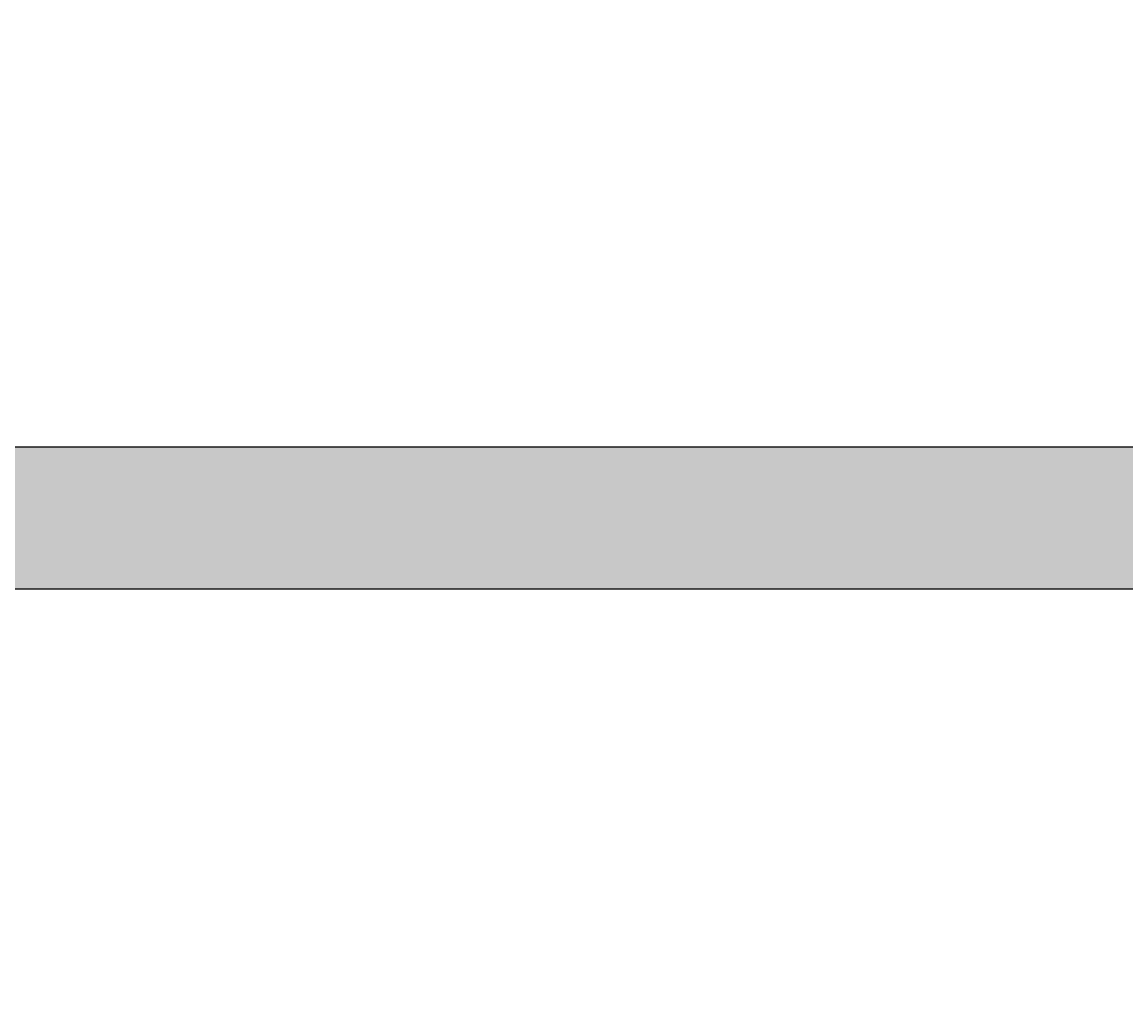
# Model space of a CAD drawing. Units: millimetres. Extents: x -11 to 280, y -4 to 208.
# Tile 21 of 55: x 91 to 119, y 61 to 85. Entities that reach past the tile are written whole.
import ezdxf

# ---------------------------------------------------------------- set-up
doc = ezdxf.new("R2010")
doc.units = ezdxf.units.MM
doc.layers.add('M-DIMS', color=2, linetype='Continuous', lineweight=18)
doc.layers.add('M-HYDR-RETN', color=7, linetype='Continuous', lineweight=25)
doc.layers.add('M-HYDR-RETN-PATT', color=114, linetype='Continuous', lineweight=13, true_color=0x139b48)
doc.styles.get("Standard").update_dxf_attribs({"font": 'arial.ttf'})
doc.dimstyles.get("Standard").update_dxf_attribs({"dimtxt": 0.18, "dimasz": 0.18, "dimexe": 0.18, "dimexo": 0.0625, "dimgap": 0.09, "dimtad": 0, "dimtih": 1, "dimtoh": 1, "dimdec": 4, "dimzin": 0, "dimdsep": 46, "dimtxsty": 'Standard', "dimcen": 0.09, "dimadec": 0, "dimazin": 0, "dimtfac": 1, "dimtdec": 4, "dimtofl": 0, "dimtmove": 0, "dimatfit": 3, "dimfxl": 1, "dimtolj": 1, "dimtzin": 0, "dimarcsym": 0})

# ---------------------------------------------------------------- blocks, each defined once
blk = doc.blocks.new('*D4')
at = {"layer": 'Defpoints', "color": 0, "transparency": 16777216}
for p in [(4.763, 84.426), (266.035, 51.733), (266.035, -3.415)]:
    blk.add_point(p, dxfattribs=at)
at = {"layer": 'M-DIMS', "color": 0, "lineweight": -2, "transparency": 16777216}
for p, q in [((4.763, 84.364), (4.763, -3.595)), ((266.035, 51.67), (266.035, -3.595)), ((4.943, -3.415), (134.934, -3.415)), ((265.855, -3.415), (135.864, -3.415))]:
    blk.add_line(p, q, dxfattribs=at)
at = {"layer": 'M-DIMS', "color": 0, "transparency": 16777216}
for points in [[(4.943, -3.385), (4.943, -3.445), (4.763, -3.415)], [(265.855, -3.385), (265.855, -3.445), (266.035, -3.415)]]:
    blk.add_solid(points, dxfattribs=at)
at = {"layer": 'M-DIMS', "color": 0, "transparency": 16777216, "insert": (135.399, -3.415), "char_height": 0.18, "attachment_point": 5}
blk.add_mtext('\\A1;261.27', dxfattribs=at)
blk = doc.blocks.new('*D5')
at = {"layer": 'Defpoints', "color": 0, "transparency": 16777216}
for p in [(24.759, 192.645), (-10.087, 11.435), (261.686, 11.435)]:
    blk.add_point(p, dxfattribs=at)
at = {"layer": 'M-DIMS', "color": 0, "lineweight": -2, "transparency": 16777216}
for p, q in [((24.696, 192.645), (-10.267, 192.645)), ((-10.087, 192.465), (-10.087, 102.222)), ((-10.087, 11.615), (-10.087, 101.858)), ((261.624, 11.435), (-10.267, 11.435))]:
    blk.add_line(p, q, dxfattribs=at)
at = {"layer": 'M-DIMS', "color": 0, "transparency": 16777216}
for points in [[(-10.117, 192.465), (-10.057, 192.465), (-10.087, 192.645)], [(-10.117, 11.615), (-10.057, 11.615), (-10.087, 11.435)]]:
    blk.add_solid(points, dxfattribs=at)
at = {"layer": 'M-DIMS', "color": 0, "transparency": 16777216, "insert": (-10.087, 102.04), "char_height": 0.18, "attachment_point": 5}
blk.add_mtext('\\A1;181.2', dxfattribs=at)

msp = doc.modelspace()

# ---------------------------------------------------------------- hatches: boundary and pattern name
at = {"layer": 'M-HYDR-RETN-PATT'}
h = msp.add_hatch(color=256, dxfattribs=at)
h.set_gradient(color1=(19, 155, 72), color2=(19, 155, 72), tint=1)
h.paths.add_polyline_path([(17.9701, 159.0814), (29.2015, 159.0814), (29.2015, 162.5814), (14.4701, 162.5814), (14.4701, 98.0213), (17.9701, 98.0213)])
h.paths.add_polyline_path([(17.9701, 84.4261), (14.4701, 84.4261), (14.4701, 54.3099), (156.2446, 54.3099), (156.2446, 57.8099), (17.9701, 57.8099)])
h.paths.add_polyline_path([(120.5137, 74.3991), (17.9701, 74.3991), (17.9701, 70.8991), (120.5137, 70.8991)], flags=17)
h.paths.add_polyline_path([(184.7092, 75.04, 0.4142136), (179.7092, 80.04), (156.2446, 80.04), (156.2446, 57.8099), (156.2446, 54.3099), (156.2446, 43.5991), (159.7446, 43.5991), (159.7446, 57.8099), (159.7446, 76.54), (176.2092, 76.54, -0.4142136), (181.2092, 71.54), (181.2092, 57.8099), (159.7446, 57.8099), (159.7446, 54.3099), (184.7092, 54.3099)])

# ---------------------------------------------------------------- linework, layer by layer
at = {"layer": 'M-HYDR-RETN'}
for points in [[(17.9701, 74.3991), (120.5137, 74.3991)], [(17.9701, 70.8991), (120.5137, 70.8991)]]:
    msp.add_lwpolyline(points, dxfattribs=at)

# ---------------------------------------------------------------- dimensions: what is measured, and where the dimension line sits
at = {"layer": 'M-DIMS'}
dim = msp.add_linear_dim(base=(-10.0865, 11.4346), p1=(24.7588, 192.645), p2=(261.6863, 11.4346), angle=90, dimstyle='Standard', override={"dimdec": 1, "dimlfac": 1, "dimrnd": 0, "dimzin": 0, "dimdsep": 46, "dimlunit": 2}, dxfattribs=at)
dim.commit()
dim.dimension.update_dxf_attribs({"geometry": '*D5', "text_midpoint": (-10.0865, 102.0398)})
dim = msp.add_linear_dim(base=(266.0352, -3.4154), p1=(4.7635, 84.4261), p2=(266.0352, 51.7328), dimstyle='Standard', override={"dimdec": 2, "dimlfac": 1, "dimrnd": 0, "dimzin": 0, "dimdsep": 46, "dimlunit": 2}, dxfattribs=at)
dim.commit()
dim.dimension.update_dxf_attribs({"geometry": '*D4', "text_midpoint": (135.3993, -3.4154)})

doc.saveas('drawing.dxf')
